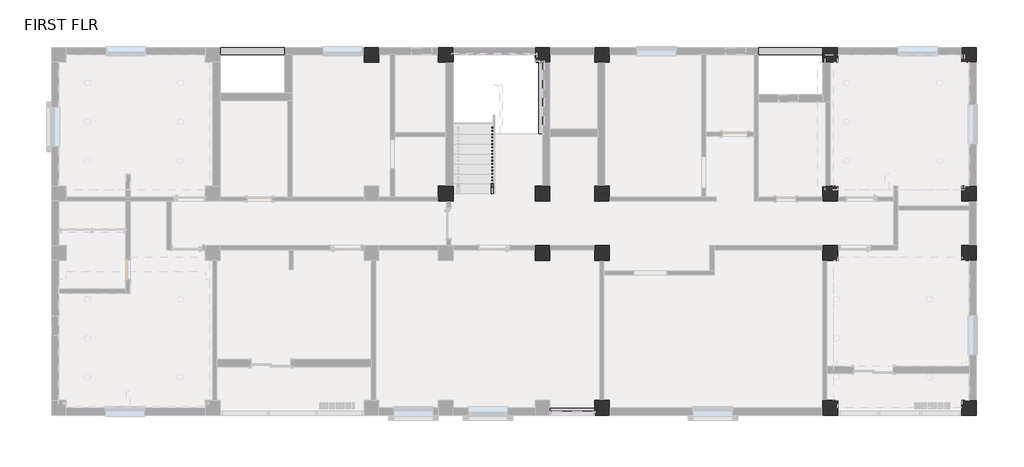
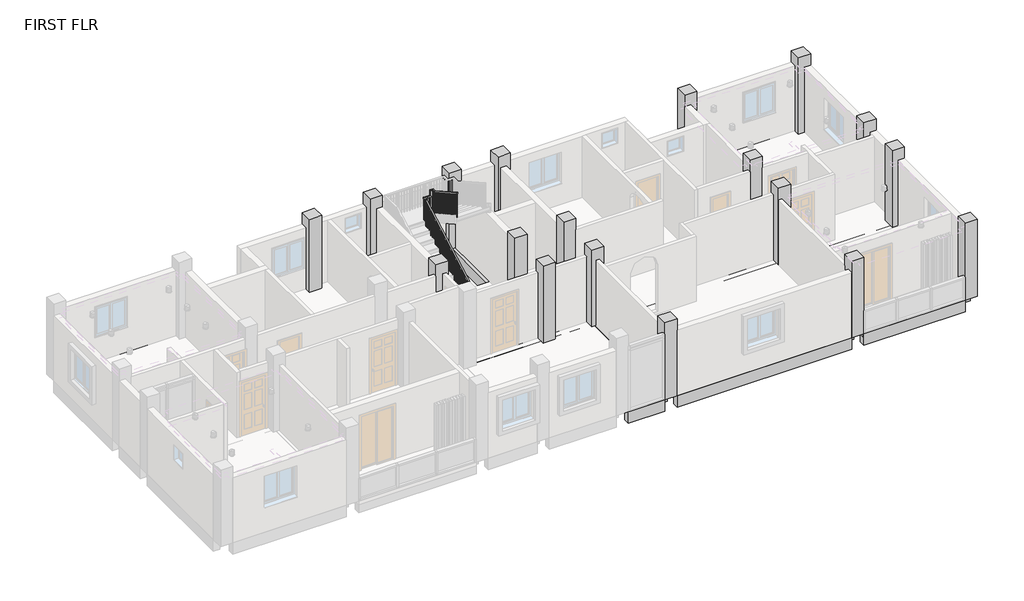
# One storey, part 4 of 5: 32 beams, 18 columns, 1 railing.
"""IFC4 building model written with IfcOpenShell, lengths in millimetres."""

from ifc_helpers import new_model, si_unit, frame, origin, place, context, project, spatial, polyline, outline, extrude, faceted_brep, element, save

model = new_model("IFC4")

# Units and contexts
model_context = context("Model", 3, world=origin())
ifc_project = project(units=[si_unit("LENGTHUNIT", "METRE", prefix="MILLI")], contexts=[model_context])

# Site, building, storey
site = spatial("IfcSite", under=ifc_project)
building = spatial("IfcBuilding", under=site)
storey = spatial("IfcBuildingStorey", under=building, Name="FIRST FLR", Elevation=3352.8)

# Beams
placement = place(None, origin())
element("IfcBeam", 1, ObjectType="Concrete-Rectangular Beam : 9\" X 18\" BEAM", at=placement, inside=storey, context=model_context, shape_type="SweptSolid", body=[
    extrude(outline(polyline([(1310.3916602, -10887.8679047), (1310.3916602, -11116.4679047), (-61.2083398, -11116.4679047), (-61.2083398, -10887.8679047), (1310.3916602, -10887.8679047)])), frame((0.0, 0.0, 2895.6), z_axis=(0.0, 0.0, 1.0), x_axis=(1.0, 0.0, 0.0)), (0.0, 0.0, 1.0), 457.2),
])
element("IfcBeam", 2, ObjectType="Concrete-Rectangular Beam : 9\" X 18\" BEAM", at=placement, inside=storey, context=model_context, shape_type="SweptSolid", body=[
    extrude(outline(polyline([(1424.6916602, -6358.3794704), (1653.2916602, -6358.3794704), (1653.2916602, -10659.2679047), (1424.6916602, -10659.2679047), (1424.6916602, -6358.3794704)])), frame((0.0, 0.0, 2895.6), z_axis=(0.0, 0.0, 1.0), x_axis=(1.0, 0.0, 0.0)), (0.0, 0.0, 1.0), 457.2),
])
element("IfcBeam", 3, ObjectType="Concrete-Rectangular Beam : 9\" X 18\" BEAM", at=placement, inside=storey, context=model_context, shape_type="SweptSolid", body=[
    extrude(outline(polyline([(1424.6916602, -4529.5794704), (1653.2916602, -4529.5794704), (1653.2916602, -5901.1794704), (1424.6916602, -5901.1794704), (1424.6916602, -4529.5794704)])), frame((0.0, 0.0, 2895.6), z_axis=(0.0, 0.0, 1.0), x_axis=(1.0, 0.0, 0.0)), (0.0, 0.0, 1.0), 457.2),
])
element("IfcBeam", 4, ObjectType="Concrete-Rectangular Beam : 9\" X 18\" BEAM", at=placement, inside=storey, context=model_context, shape_type="SweptSolid", body=[
    extrude(outline(polyline([(8317.2128058, -10887.8679047), (8317.2128058, -11116.4679047), (1767.5916602, -11116.4679047), (1767.5916602, -10887.8679047), (8317.2128058, -10887.8679047)])), frame((0.0, 0.0, 2895.6), z_axis=(0.0, 0.0, 1.0), x_axis=(1.0, 0.0, 0.0)), (0.0, 0.0, 1.0), 457.2),
])
element("IfcBeam", 5, ObjectType="Concrete-Rectangular Beam : 9\" X 18\" BEAM", at=placement, inside=storey, context=model_context, shape_type="SweptSolid", body=[
    extrude(outline(polyline([(12584.4128058, -10887.8679047), (12584.4128058, -11116.4679047), (8774.4128058, -11116.4679047), (8774.4128058, -10887.8679047), (12584.4128058, -10887.8679047)])), frame((0.0, 0.0, 2895.6), z_axis=(0.0, 0.0, 1.0), x_axis=(1.0, 0.0, 0.0)), (0.0, 0.0, 1.0), 457.2),
])
element("IfcBeam", 6, ObjectType="Concrete-Rectangular Beam : 9\" X 18\" BEAM", at=placement, inside=storey, context=model_context, shape_type="SweptSolid", body=[
    extrude(outline(polyline([(12813.0128058, -6358.3794704), (13041.6128058, -6358.3794704), (13041.6128058, -10659.2679047), (12813.0128058, -10659.2679047), (12813.0128058, -6358.3794704)])), frame((0.0, 0.0, 2895.6), z_axis=(0.0, 0.0, 1.0), x_axis=(1.0, 0.0, 0.0)), (0.0, 0.0, 1.0), 457.2),
])
element("IfcBeam", 7, ObjectType="Concrete-Rectangular Beam : 9\" X 18\" BEAM", at=placement, inside=storey, context=model_context, shape_type="SweptSolid", body=[
    extrude(outline(polyline([(12813.0128058, -4529.5794704), (13041.6128058, -4529.5794704), (13041.6128058, -5901.1794704), (12813.0128058, -5901.1794704), (12813.0128058, -4529.5794704)])), frame((0.0, 0.0, 2895.6), z_axis=(0.0, 0.0, 1.0), x_axis=(1.0, 0.0, 0.0)), (0.0, 0.0, 1.0), 457.2),
])
element("IfcBeam", 8, ObjectType="Concrete-Rectangular Beam : 9\" X 18\" BEAM", at=placement, inside=storey, context=model_context, shape_type="SweptSolid", body=[
    extrude(outline(polyline([(12813.0128058, -262.3794704), (13041.6128058, -262.3794704), (13041.6128058, -4072.3794704), (12813.0128058, -4072.3794704), (12813.0128058, -262.3794704)])), frame((0.0, 0.0, 2895.6), z_axis=(0.0, 0.0, 1.0), x_axis=(1.0, 0.0, 0.0)), (0.0, 0.0, 1.0), 457.2),
])
element("IfcBeam", 9, ObjectType="Concrete-Rectangular Beam : 9\" X 18\" BEAM", at=placement, inside=storey, context=model_context, shape_type="SweptSolid", body=[
    extrude(outline(polyline([(8774.4128058, -33.7794704), (8774.4128058, 194.8205296), (12584.4128058, 194.8205296), (12584.4128058, -33.7794704), (8774.4128058, -33.7794704)])), frame((0.0, 0.0, 2895.6), z_axis=(0.0, 0.0, 1.0), x_axis=(1.0, 0.0, 0.0)), (0.0, 0.0, 1.0), 457.2),
])
element("IfcBeam", 10, ObjectType="Concrete-Rectangular Beam : 9\" X 18\" BEAM", at=placement, inside=storey, context=model_context, shape_type="SweptSolid", body=[
    extrude(outline(polyline([(1767.5916602, -33.7794704), (1767.5916602, 194.8205296), (8317.2128058, 194.8205296), (8317.2128058, -33.7794704), (1767.5916602, -33.7794704)])), frame((0.0, 0.0, 2895.6), z_axis=(0.0, 0.0, 1.0), x_axis=(1.0, 0.0, 0.0)), (0.0, 0.0, 1.0), 457.2),
])
element("IfcBeam", 11, ObjectType="Concrete-Rectangular Beam : 9\" X 18\" BEAM", at=placement, inside=storey, context=model_context, shape_type="SweptSolid", body=[
    extrude(outline(polyline([(-61.2083398, -33.7794704), (-61.2083398, 194.8205296), (1310.3916602, 194.8205296), (1310.3916602, -33.7794704), (-61.2083398, -33.7794704)])), frame((0.0, 0.0, 2895.6), z_axis=(0.0, 0.0, 1.0), x_axis=(1.0, 0.0, 0.0)), (0.0, 0.0, 1.0), 457.2),
])
element("IfcBeam", 12, ObjectType="Concrete-Rectangular Beam : 9\" X 18\" BEAM", at=placement, inside=storey, context=model_context, shape_type="SweptSolid", body=[
    extrude(outline(polyline([(-3029.5456086, -33.7794704), (-3029.5456086, 194.8205296), (-518.4083398, 194.8205296), (-518.4083398, -33.7794704), (-3029.5456086, -33.7794704)])), frame((0.0, 0.0, 2895.6), z_axis=(0.0, 0.0, 1.0), x_axis=(1.0, 0.0, 0.0)), (0.0, 0.0, 1.0), 457.2),
])
element("IfcBeam", 13, ObjectType="Concrete-Rectangular Beam : 9\" X 18\" BEAM", at=placement, inside=storey, context=model_context, shape_type="SweptSolid", body=[
    extrude(outline(polyline([(-5315.5456086, -33.7794704), (-5315.5456086, 194.8205296), (-3486.7456086, 194.8205296), (-3486.7456086, -33.7794704), (-5315.5456086, -33.7794704)])), frame((0.0, 0.0, 2895.6), z_axis=(0.0, 0.0, 1.0), x_axis=(1.0, 0.0, 0.0)), (0.0, 0.0, 1.0), 457.2),
])
element("IfcBeam", 14, ObjectType="Concrete-Rectangular Beam : 9\" X 18\" BEAM", at=placement, inside=storey, context=model_context, shape_type="SweptSolid", body=[
    extrude(outline(polyline([(-10192.3456086, -33.7794704), (-10192.3456086, 194.8205296), (-5772.7456086, 194.8205296), (-5772.7456086, -33.7794704), (-10192.3456086, -33.7794704)])), frame((0.0, 0.0, 2895.6), z_axis=(0.0, 0.0, 1.0), x_axis=(1.0, 0.0, 0.0)), (0.0, 0.0, 1.0), 457.2),
])
element("IfcBeam", 15, ObjectType="Concrete-Rectangular Beam : 9\" X 18\" BEAM", at=placement, inside=storey, context=model_context, shape_type="SweptSolid", body=[
    extrude(outline(polyline([(-14916.7456086, -33.7794704), (-14916.7456086, 194.8205296), (-10649.5456086, 194.8205296), (-10649.5456086, -33.7794704), (-14916.7456086, -33.7794704)])), frame((0.0, 0.0, 2895.6), z_axis=(0.0, 0.0, 1.0), x_axis=(1.0, 0.0, 0.0)), (0.0, 0.0, 1.0), 457.2),
])
element("IfcBeam", 16, ObjectType="Concrete-Rectangular Beam : 9\" X 18\" BEAM", at=placement, inside=storey, context=model_context, shape_type="SweptSolid", body=[
    extrude(outline(polyline([(-518.4083398, -4186.6794704), (-518.4083398, -4415.2794704), (-3029.5456086, -4415.2794704), (-3029.5456086, -4186.6794704), (-518.4083398, -4186.6794704)])), frame((0.0, 0.0, 2895.6), z_axis=(0.0, 0.0, 1.0), x_axis=(1.0, 0.0, 0.0)), (0.0, 0.0, 1.0), 457.2),
])
element("IfcBeam", 17, ObjectType="Concrete-Rectangular Beam : 9\" X 18\" BEAM", at=placement, inside=storey, context=model_context, shape_type="SweptSolid", body=[
    extrude(outline(polyline([(1310.3916602, -4186.6794704), (1310.3916602, -4415.2794704), (-61.2083398, -4415.2794704), (-61.2083398, -4186.6794704), (1310.3916602, -4186.6794704)])), frame((0.0, 0.0, 2895.6), z_axis=(0.0, 0.0, 1.0), x_axis=(1.0, 0.0, 0.0)), (0.0, 0.0, 1.0), 457.2),
])
element("IfcBeam", 18, ObjectType="Concrete-Rectangular Beam : 9\" X 18\" BEAM", at=placement, inside=storey, context=model_context, shape_type="SweptSolid", body=[
    extrude(outline(polyline([(1424.6916602, -262.3794704), (1653.2916602, -262.3794704), (1653.2916602, -4072.3794704), (1424.6916602, -4072.3794704), (1424.6916602, -262.3794704)])), frame((0.0, 0.0, 2895.6), z_axis=(0.0, 0.0, 1.0), x_axis=(1.0, 0.0, 0.0)), (0.0, 0.0, 1.0), 457.2),
])
element("IfcBeam", 19, ObjectType="Concrete-Rectangular Beam : 9\" X 18\" BEAM", at=placement, inside=storey, context=model_context, shape_type="SweptSolid", body=[
    extrude(outline(polyline([(-175.5083398, -4072.3794704), (-404.1083398, -4072.3794704), (-404.1083398, -262.3794704), (-175.5083398, -262.3794704), (-175.5083398, -4072.3794704)])), frame((0.0, 0.0, 2895.6), z_axis=(0.0, 0.0, 1.0), x_axis=(1.0, 0.0, 0.0)), (0.0, 0.0, 1.0), 457.2),
])
element("IfcBeam", 20, ObjectType="Concrete-Rectangular Beam : 9\" X 18\" BEAM", at=placement, inside=storey, context=model_context, shape_type="SweptSolid", body=[
    extrude(outline(polyline([(-3143.8456086, -4072.3794704), (-3372.4456086, -4072.3794704), (-3372.4456086, -262.3794704), (-3143.8456086, -262.3794704), (-3143.8456086, -4072.3794704)])), frame((0.0, 0.0, 2895.6), z_axis=(0.0, 0.0, 1.0), x_axis=(1.0, 0.0, 0.0)), (0.0, 0.0, 1.0), 457.2),
])
element("IfcBeam", 21, ObjectType="Concrete-Rectangular Beam : 9\" X 18\" BEAM", at=placement, inside=storey, context=model_context, shape_type="SweptSolid", body=[
    extrude(outline(polyline([(-5429.8456086, -4072.3794704), (-5658.4456086, -4072.3794704), (-5658.4456086, -262.3794704), (-5429.8456086, -262.3794704), (-5429.8456086, -4072.3794704)])), frame((0.0, 0.0, 2895.6), z_axis=(0.0, 0.0, 1.0), x_axis=(1.0, 0.0, 0.0)), (0.0, 0.0, 1.0), 457.2),
])
element("IfcBeam", 22, ObjectType="Concrete-Rectangular Beam : 9\" X 18\" BEAM", at=placement, inside=storey, context=model_context, shape_type="SweptSolid", body=[
    extrude(outline(polyline([(-3029.5456086, -6244.0794704), (-3029.5456086, -6015.4794704), (-518.4083398, -6015.4794704), (-518.4083398, -6244.0794704), (-3029.5456086, -6244.0794704)])), frame((0.0, 0.0, 2895.6), z_axis=(0.0, 0.0, 1.0), x_axis=(1.0, 0.0, 0.0)), (0.0, 0.0, 1.0), 457.2),
])
element("IfcBeam", 23, ObjectType="Concrete-Rectangular Beam : 9\" X 18\" BEAM", at=placement, inside=storey, context=model_context, shape_type="SweptSolid", body=[
    extrude(outline(polyline([(1310.3916602, -6015.4794704), (1310.3916602, -6244.0794704), (-61.2083398, -6244.0794704), (-61.2083398, -6015.4794704), (1310.3916602, -6015.4794704)])), frame((0.0, 0.0, 2895.6), z_axis=(0.0, 0.0, 1.0), x_axis=(1.0, 0.0, 0.0)), (0.0, 0.0, 1.0), 457.2),
])
element("IfcBeam", 24, ObjectType="Concrete-Rectangular Beam : 9\" X 18\" BEAM", at=placement, inside=storey, context=model_context, shape_type="SweptSolid", body=[
    extrude(outline(polyline([(-404.1083398, -4529.5794704), (-175.5083398, -4529.5794704), (-175.5083398, -5901.1794704), (-404.1083398, -5901.1794704), (-404.1083398, -4529.5794704)])), frame((0.0, 0.0, 2895.6), z_axis=(0.0, 0.0, 1.0), x_axis=(1.0, 0.0, 0.0)), (0.0, 0.0, 1.0), 457.2),
])
element("IfcBeam", 25, ObjectType="Concrete-Rectangular Beam : 9\" X 18\" BEAM", at=placement, inside=storey, context=model_context, shape_type="SweptSolid", body=[
    extrude(outline(polyline([(-3143.8456086, -5901.1794704), (-3372.4456086, -5901.1794704), (-3372.4456086, -4529.5794704), (-3143.8456086, -4529.5794704), (-3143.8456086, -5901.1794704)])), frame((0.0, 0.0, 2895.6), z_axis=(0.0, 0.0, 1.0), x_axis=(1.0, 0.0, 0.0)), (0.0, 0.0, 1.0), 457.2),
])
element("IfcBeam", 26, ObjectType="Concrete-Rectangular Beam : 9\" X 18\" BEAM", at=placement, inside=storey, context=model_context, shape_type="SweptSolid", body=[
    extrude(outline(polyline([(8317.2128058, -4186.6794704), (8317.2128058, -4415.2794704), (1767.5916602, -4415.2794704), (1767.5916602, -4186.6794704), (8317.2128058, -4186.6794704)])), frame((0.0, 0.0, 2895.6), z_axis=(0.0, 0.0, 1.0), x_axis=(1.0, 0.0, 0.0)), (0.0, 0.0, 1.0), 457.2),
])
element("IfcBeam", 27, ObjectType="Concrete-Rectangular Beam : 9\" X 18\" BEAM", at=placement, inside=storey, context=model_context, shape_type="SweptSolid", body=[
    extrude(outline(polyline([(12584.4128058, -4186.6794704), (12584.4128058, -4415.2794704), (8774.4128058, -4415.2794704), (8774.4128058, -4186.6794704), (12584.4128058, -4186.6794704)])), frame((0.0, 0.0, 2895.6), z_axis=(0.0, 0.0, 1.0), x_axis=(1.0, 0.0, 0.0)), (0.0, 0.0, 1.0), 457.2),
])
element("IfcBeam", 28, ObjectType="Concrete-Rectangular Beam : 9\" X 18\" BEAM", at=placement, inside=storey, context=model_context, shape_type="SweptSolid", body=[
    extrude(outline(polyline([(8774.4128058, -6244.0794704), (8774.4128058, -6015.4794704), (12584.4128058, -6015.4794704), (12584.4128058, -6244.0794704), (8774.4128058, -6244.0794704)])), frame((0.0, 0.0, 2895.6), z_axis=(0.0, 0.0, 1.0), x_axis=(1.0, 0.0, 0.0)), (0.0, 0.0, 1.0), 457.2),
])
element("IfcBeam", 29, ObjectType="Concrete-Rectangular Beam : 9\" X 18\" BEAM", at=placement, inside=storey, context=model_context, shape_type="SweptSolid", body=[
    extrude(outline(polyline([(1767.5916602, -6244.0794704), (1767.5916602, -6015.4794704), (8317.2128058, -6015.4794704), (8317.2128058, -6244.0794704), (1767.5916602, -6244.0794704)])), frame((0.0, 0.0, 2895.6), z_axis=(0.0, 0.0, 1.0), x_axis=(1.0, 0.0, 0.0)), (0.0, 0.0, 1.0), 457.2),
])
element("IfcBeam", 30, ObjectType="Concrete-Rectangular Beam : 9\" X 18\" BEAM", at=placement, inside=storey, context=model_context, shape_type="SweptSolid", body=[
    extrude(outline(polyline([(8431.5128058, -6358.3794704), (8660.1128058, -6358.3794704), (8660.1128058, -10659.2679047), (8431.5128058, -10659.2679047), (8431.5128058, -6358.3794704)])), frame((0.0, 0.0, 2895.6), z_axis=(0.0, 0.0, 1.0), x_axis=(1.0, 0.0, 0.0)), (0.0, 0.0, 1.0), 457.2),
])
element("IfcBeam", 31, ObjectType="Concrete-Rectangular Beam : 9\" X 18\" BEAM", at=placement, inside=storey, context=model_context, shape_type="SweptSolid", body=[
    extrude(outline(polyline([(8431.5128058, -4529.5794704), (8660.1128058, -4529.5794704), (8660.1128058, -5901.1794704), (8431.5128058, -5901.1794704), (8431.5128058, -4529.5794704)])), frame((0.0, 0.0, 2895.6), z_axis=(0.0, 0.0, 1.0), x_axis=(1.0, 0.0, 0.0)), (0.0, 0.0, 1.0), 457.2),
])
element("IfcBeam", 32, ObjectType="Concrete-Rectangular Beam : 9\" X 18\" BEAM", at=placement, inside=storey, context=model_context, shape_type="SweptSolid", body=[
    extrude(outline(polyline([(8431.5128058, -262.3794704), (8660.1128058, -262.3794704), (8660.1128058, -4072.3794704), (8431.5128058, -4072.3794704), (8431.5128058, -262.3794704)])), frame((0.0, 0.0, 2895.6), z_axis=(0.0, 0.0, 1.0), x_axis=(1.0, 0.0, 0.0)), (0.0, 0.0, 1.0), 457.2),
])

# Columns
element("IfcColumn", 33, ObjectType="Concrete-Rectangular-Column : COLUMN 18\" X 18\"", at=placement, inside=storey, context=model_context, shape_type="SweptSolid", body=[
    extrude(outline(polyline([(-5315.5456086, 194.8205296), (-5315.5456086, -262.3794704), (-5772.7456086, -262.3794704), (-5772.7456086, 194.8205296), (-5315.5456086, 194.8205296)])), frame((0.0, 0.0, 3352.8), z_axis=(0.0, 0.0, 1.0), x_axis=(1.0, 0.0, 0.0)), (0.0, 0.0, 1.0), 3048.0),
])
element("IfcColumn", 34, ObjectType="Concrete-Rectangular-Column : COLUMN 18\" X 18\"", at=placement, inside=storey, context=model_context, shape_type="SweptSolid", body=[
    extrude(outline(polyline([(-3029.5456086, 194.8205296), (-3029.5456086, -262.3794704), (-3486.7456086, -262.3794704), (-3486.7456086, 194.8205296), (-3029.5456086, 194.8205296)])), frame((0.0, 0.0, 3352.8), z_axis=(0.0, 0.0, 1.0), x_axis=(1.0, 0.0, 0.0)), (0.0, 0.0, 1.0), 3048.0),
])
element("IfcColumn", 35, ObjectType="Concrete-Rectangular-Column : COLUMN 18\" X 18\"", at=placement, inside=storey, context=model_context, shape_type="SweptSolid", body=[
    extrude(outline(polyline([(-61.2083398, 194.8205296), (-61.2083398, -262.3794704), (-518.4083398, -262.3794704), (-518.4083398, 194.8205296), (-61.2083398, 194.8205296)])), frame((0.0, 0.0, 3352.8), z_axis=(0.0, 0.0, 1.0), x_axis=(1.0, 0.0, 0.0)), (0.0, 0.0, 1.0), 3048.0),
])
element("IfcColumn", 36, ObjectType="Concrete-Rectangular-Column : COLUMN 18\" X 18\"", at=placement, inside=storey, context=model_context, shape_type="SweptSolid", body=[
    extrude(outline(polyline([(1767.5916602, 194.8205296), (1767.5916602, -262.3794704), (1310.3916602, -262.3794704), (1310.3916602, 194.8205296), (1767.5916602, 194.8205296)])), frame((0.0, 0.0, 3352.8), z_axis=(0.0, 0.0, 1.0), x_axis=(1.0, 0.0, 0.0)), (0.0, 0.0, 1.0), 3048.0),
])
element("IfcColumn", 37, ObjectType="Concrete-Rectangular-Column : COLUMN 18\" X 18\"", at=placement, inside=storey, context=model_context, shape_type="SweptSolid", body=[
    extrude(outline(polyline([(8774.4128058, 194.8205296), (8774.4128058, -262.3794704), (8317.2128058, -262.3794704), (8317.2128058, 194.8205296), (8774.4128058, 194.8205296)])), frame((0.0, 0.0, 3352.8), z_axis=(0.0, 0.0, 1.0), x_axis=(1.0, 0.0, 0.0)), (0.0, 0.0, 1.0), 3048.0),
])
element("IfcColumn", 38, ObjectType="Concrete-Rectangular-Column : COLUMN 18\" X 18\"", at=placement, inside=storey, context=model_context, shape_type="SweptSolid", body=[
    extrude(outline(polyline([(13041.6128058, 194.8205296), (13041.6128058, -262.3794704), (12584.4128058, -262.3794704), (12584.4128058, 194.8205296), (13041.6128058, 194.8205296)])), frame((0.0, 0.0, 3352.8), z_axis=(0.0, 0.0, 1.0), x_axis=(1.0, 0.0, 0.0)), (0.0, 0.0, 1.0), 3048.0),
])
element("IfcColumn", 39, ObjectType="Concrete-Rectangular-Column : COLUMN 18\" X 18\"", at=placement, inside=storey, context=model_context, shape_type="SweptSolid", body=[
    extrude(outline(polyline([(13041.6128058, -4072.3794704), (13041.6128058, -4529.5794704), (12584.4128058, -4529.5794704), (12584.4128058, -4072.3794704), (13041.6128058, -4072.3794704)])), frame((0.0, 0.0, 3352.8), z_axis=(0.0, 0.0, 1.0), x_axis=(1.0, 0.0, 0.0)), (0.0, 0.0, 1.0), 3048.0),
])
element("IfcColumn", 40, ObjectType="Concrete-Rectangular-Column : COLUMN 18\" X 18\"", at=placement, inside=storey, context=model_context, shape_type="SweptSolid", body=[
    extrude(outline(polyline([(13041.6128058, -5901.1794704), (13041.6128058, -6358.3794704), (12584.4128058, -6358.3794704), (12584.4128058, -5901.1794704), (13041.6128058, -5901.1794704)])), frame((0.0, 0.0, 3352.8), z_axis=(0.0, 0.0, 1.0), x_axis=(1.0, 0.0, 0.0)), (0.0, 0.0, 1.0), 3048.0),
])
element("IfcColumn", 41, ObjectType="Concrete-Rectangular-Column : COLUMN 18\" X 18\"", at=placement, inside=storey, context=model_context, shape_type="SweptSolid", body=[
    extrude(outline(polyline([(13041.6128058, -10659.2679047), (13041.6128058, -11116.4679047), (12584.4128058, -11116.4679047), (12584.4128058, -10659.2679047), (13041.6128058, -10659.2679047)])), frame((0.0, 0.0, 3352.8), z_axis=(0.0, 0.0, 1.0), x_axis=(1.0, 0.0, 0.0)), (0.0, 0.0, 1.0), 3048.0),
])
element("IfcColumn", 42, ObjectType="Concrete-Rectangular-Column : COLUMN 18\" X 18\"", at=placement, inside=storey, context=model_context, shape_type="SweptSolid", body=[
    extrude(outline(polyline([(8774.4128058, -10659.2679047), (8774.4128058, -11116.4679047), (8317.2128058, -11116.4679047), (8317.2128058, -10659.2679047), (8774.4128058, -10659.2679047)])), frame((0.0, 0.0, 3352.8), z_axis=(0.0, 0.0, 1.0), x_axis=(1.0, 0.0, 0.0)), (0.0, 0.0, 1.0), 3048.0),
])
element("IfcColumn", 43, ObjectType="Concrete-Rectangular-Column : COLUMN 18\" X 18\"", at=placement, inside=storey, context=model_context, shape_type="SweptSolid", body=[
    extrude(outline(polyline([(1767.5916602, -10659.2679047), (1767.5916602, -11116.4679047), (1310.3916602, -11116.4679047), (1310.3916602, -10659.2679047), (1767.5916602, -10659.2679047)])), frame((0.0, 0.0, 3352.8), z_axis=(0.0, 0.0, 1.0), x_axis=(1.0, 0.0, 0.0)), (0.0, 0.0, 1.0), 3048.0),
])
element("IfcColumn", 44, ObjectType="Concrete-Rectangular-Column : COLUMN 18\" X 18\"", at=placement, inside=storey, context=model_context, shape_type="SweptSolid", body=[
    extrude(outline(polyline([(-3029.5456086, -4072.3794704), (-3029.5456086, -4529.5794704), (-3486.7456086, -4529.5794704), (-3486.7456086, -4072.3794704), (-3029.5456086, -4072.3794704)])), frame((0.0, 0.0, 3352.8), z_axis=(0.0, 0.0, 1.0), x_axis=(1.0, 0.0, 0.0)), (0.0, 0.0, 1.0), 3048.0),
])
element("IfcColumn", 45, ObjectType="Concrete-Rectangular-Column : COLUMN 18\" X 18\"", at=placement, inside=storey, context=model_context, shape_type="SweptSolid", body=[
    extrude(outline(polyline([(-61.2083398, -4072.3794704), (-61.2083398, -4529.5794704), (-518.4083398, -4529.5794704), (-518.4083398, -4072.3794704), (-61.2083398, -4072.3794704)])), frame((0.0, 0.0, 3352.8), z_axis=(0.0, 0.0, 1.0), x_axis=(1.0, 0.0, 0.0)), (0.0, 0.0, 1.0), 3048.0),
])
element("IfcColumn", 46, ObjectType="Concrete-Rectangular-Column : COLUMN 18\" X 18\"", at=placement, inside=storey, context=model_context, shape_type="SweptSolid", body=[
    extrude(outline(polyline([(1767.5916602, -4072.3794704), (1767.5916602, -4529.5794704), (1310.3916602, -4529.5794704), (1310.3916602, -4072.3794704), (1767.5916602, -4072.3794704)])), frame((0.0, 0.0, 3352.8), z_axis=(0.0, 0.0, 1.0), x_axis=(1.0, 0.0, 0.0)), (0.0, 0.0, 1.0), 3048.0),
])
element("IfcColumn", 47, ObjectType="Concrete-Rectangular-Column : COLUMN 18\" X 18\"", at=placement, inside=storey, context=model_context, shape_type="SweptSolid", body=[
    extrude(outline(polyline([(8774.4128058, -4072.3794704), (8774.4128058, -4529.5794704), (8317.2128058, -4529.5794704), (8317.2128058, -4072.3794704), (8774.4128058, -4072.3794704)])), frame((0.0, 0.0, 3352.8), z_axis=(0.0, 0.0, 1.0), x_axis=(1.0, 0.0, 0.0)), (0.0, 0.0, 1.0), 3048.0),
])
element("IfcColumn", 48, ObjectType="Concrete-Rectangular-Column : COLUMN 18\" X 18\"", at=placement, inside=storey, context=model_context, shape_type="SweptSolid", body=[
    extrude(outline(polyline([(8774.4128058, -5901.1794704), (8774.4128058, -6358.3794704), (8317.2128058, -6358.3794704), (8317.2128058, -5901.1794704), (8774.4128058, -5901.1794704)])), frame((0.0, 0.0, 3352.8), z_axis=(0.0, 0.0, 1.0), x_axis=(1.0, 0.0, 0.0)), (0.0, 0.0, 1.0), 3048.0),
])
element("IfcColumn", 49, ObjectType="Concrete-Rectangular-Column : COLUMN 18\" X 18\"", at=placement, inside=storey, context=model_context, shape_type="SweptSolid", body=[
    extrude(outline(polyline([(1767.5916602, -5901.1794704), (1767.5916602, -6358.3794704), (1310.3916602, -6358.3794704), (1310.3916602, -5901.1794704), (1767.5916602, -5901.1794704)])), frame((0.0, 0.0, 3352.8), z_axis=(0.0, 0.0, 1.0), x_axis=(1.0, 0.0, 0.0)), (0.0, 0.0, 1.0), 3048.0),
])
element("IfcColumn", 50, ObjectType="Concrete-Rectangular-Column : COLUMN 18\" X 18\"", at=placement, inside=storey, context=model_context, shape_type="SweptSolid", body=[
    extrude(outline(polyline([(-61.2083398, -5901.1794704), (-61.2083398, -6358.3794704), (-518.4083398, -6358.3794704), (-518.4083398, -5901.1794704), (-61.2083398, -5901.1794704)])), frame((0.0, 0.0, 3352.8), z_axis=(0.0, 0.0, 1.0), x_axis=(1.0, 0.0, 0.0)), (0.0, 0.0, 1.0), 3048.0),
])

# Railing
element("IfcRailing", 51, ObjectType="Handrail - Rectangular", at=placement, inside=storey, context=model_context, shape_type="SolidModel", body=[
    faceted_brep([(-1861.1456086, -4300.9794704, 4436.5333333), (-1861.1456086, -4300.9794704, 4378.420221), (-1810.3456086, -4300.9794704, 4378.420221), (-1810.3456086, -4300.9794704, 4436.5333333), (-1861.1456086, -1024.3794704, 6256.8666667), (-1861.1456086, -973.5794704, 6226.9757765), (-1810.3456086, -973.5794704, 6226.9757765), (-1810.3456086, -1024.3794704, 6256.8666667), (-1861.1456086, -1024.3794704, 6299.2), (-1861.1456086, -973.5794704, 6248.4), (-1810.3456086, -973.5794704, 6248.4), (-1810.3456086, -1024.3794704, 6299.2), (-1861.1456086, -897.3794704, 6299.2), (-1861.1456086, -897.3794704, 6248.4), (-1810.3456086, -948.1794704, 6248.4), (-1810.3456086, -948.1794704, 6299.2), (-1734.1456086, -897.3794704, 6299.2), (-1734.1456086, -897.3794704, 6248.4), (-1734.1456086, -948.1794704, 6248.4), (-1734.1456086, -948.1794704, 6299.2), (-1610.6083398, -897.3794704, 6299.2), (-1559.8083398, -897.3794704, 6248.4), (-1559.8083398, -948.1794704, 6248.4), (-1610.6083398, -948.1794704, 6299.2), (-1610.6083398, -897.3794704, 6510.8666667), (-1559.8083398, -897.3794704, 6460.0666667), (-1559.8083398, -948.1794704, 6460.0666667), (-1610.6083398, -948.1794704, 6510.8666667), (-1483.6083398, -897.3794704, 6510.8666667), (-1483.6083398, -897.3794704, 6460.0666667), (-1534.4083398, -948.1794704, 6460.0666667), (-1534.4083398, -948.1794704, 6510.8666667), (-1483.6083398, -1024.3794704, 6510.8666667), (-1483.6083398, -1037.5430727, 6460.0666667), (-1534.4083398, -1037.5430727, 6460.0666667), (-1534.4083398, -1024.3794704, 6510.8666667), (-1483.6083398, -2472.1794704, 7315.2), (-1534.4083398, -2472.1794704, 7315.2), (-1534.4083398, -2472.1794704, 7257.0868876), (-1483.6083398, -2472.1794704, 7257.0868876)], [[[0, 1, 2, 3]], [[1, 0, 4, 5]], [[2, 1, 5, 6]], [[3, 2, 6, 7]], [[0, 3, 7, 4]], [[5, 4, 8, 9]], [[6, 5, 9, 10]], [[7, 6, 10, 11]], [[4, 7, 11, 8]], [[9, 8, 12, 13]], [[10, 9, 13, 14]], [[11, 10, 14, 15]], [[8, 11, 15, 12]], [[13, 12, 16, 17]], [[14, 13, 17, 18]], [[15, 14, 18, 19]], [[12, 15, 19, 16]], [[17, 16, 20, 21]], [[18, 17, 21, 22]], [[19, 18, 22, 23]], [[16, 19, 23, 20]], [[21, 20, 24, 25]], [[22, 21, 25, 26]], [[23, 22, 26, 27]], [[20, 23, 27, 24]], [[25, 24, 28, 29]], [[26, 25, 29, 30]], [[27, 26, 30, 31]], [[24, 27, 31, 28]], [[29, 28, 32, 33]], [[30, 29, 33, 34]], [[31, 30, 34, 35]], [[28, 31, 35, 32]], [[36, 37, 38, 39]], [[33, 32, 36, 39]], [[34, 33, 39, 38]], [[35, 34, 38, 37]], [[32, 35, 37, 36]]]),
    extrude(outline(polyline([(-2456.3044704, 7248.2674432), (-2437.2544704, 7237.6841099), (-2437.2544704, 6231.4666667), (-2456.3044704, 6231.4666667), (-2456.3044704, 7248.2674432)])), frame((-1518.5333398, 0.0, 0.0), z_axis=(1.0, 0.0, 0.0), x_axis=(0.0, 1.0, 0.0)), (0.0, 0.0, 1.0), 19.05),
    extrude(outline(polyline([(-2354.7044704, 7191.8229988), (-2335.6544704, 7181.2396654), (-2335.6544704, 6231.4666667), (-2354.7044704, 6231.4666667), (-2354.7044704, 7191.8229988)])), frame((-1518.5333398, 0.0, 0.0), z_axis=(1.0, 0.0, 0.0), x_axis=(0.0, 1.0, 0.0)), (0.0, 0.0, 1.0), 19.05),
    extrude(outline(polyline([(-2253.1044704, 7135.3785543), (-2234.0544704, 7124.795221), (-2234.0544704, 6231.4666667), (-2253.1044704, 6231.4666667), (-2253.1044704, 7135.3785543)])), frame((-1518.5333398, 0.0, 0.0), z_axis=(1.0, 0.0, 0.0), x_axis=(0.0, 1.0, 0.0)), (0.0, 0.0, 1.0), 19.05),
    extrude(outline(polyline([(-2151.5044704, 7078.9341099), (-2132.4544704, 7068.3507765), (-2132.4544704, 6062.1333333), (-2151.5044704, 6062.1333333), (-2151.5044704, 7078.9341099)])), frame((-1518.5333398, 0.0, 0.0), z_axis=(1.0, 0.0, 0.0), x_axis=(0.0, 1.0, 0.0)), (0.0, 0.0, 1.0), 19.05),
    extrude(outline(polyline([(-2049.9044704, 7022.4896654), (-2030.8544704, 7011.9063321), (-2030.8544704, 6062.1333333), (-2049.9044704, 6062.1333333), (-2049.9044704, 7022.4896654)])), frame((-1518.5333398, 0.0, 0.0), z_axis=(1.0, 0.0, 0.0), x_axis=(0.0, 1.0, 0.0)), (0.0, 0.0, 1.0), 19.05),
    extrude(outline(polyline([(-1948.3044704, 6966.045221), (-1929.2544704, 6955.4618876), (-1929.2544704, 6062.1333333), (-1948.3044704, 6062.1333333), (-1948.3044704, 6966.045221)])), frame((-1518.5333398, 0.0, 0.0), z_axis=(1.0, 0.0, 0.0), x_axis=(0.0, 1.0, 0.0)), (0.0, 0.0, 1.0), 19.05),
    extrude(outline(polyline([(-1846.7044704, 6909.6007765), (-1827.6544704, 6899.0174432), (-1827.6544704, 5892.8), (-1846.7044704, 5892.8), (-1846.7044704, 6909.6007765)])), frame((-1518.5333398, 0.0, 0.0), z_axis=(1.0, 0.0, 0.0), x_axis=(0.0, 1.0, 0.0)), (0.0, 0.0, 1.0), 19.05),
    extrude(outline(polyline([(-1745.1044704, 6853.1563321), (-1726.0544704, 6842.5729988), (-1726.0544704, 5892.8), (-1745.1044704, 5892.8), (-1745.1044704, 6853.1563321)])), frame((-1518.5333398, 0.0, 0.0), z_axis=(1.0, 0.0, 0.0), x_axis=(0.0, 1.0, 0.0)), (0.0, 0.0, 1.0), 19.05),
    extrude(outline(polyline([(-1643.5044704, 6796.7118876), (-1624.4544704, 6786.1285543), (-1624.4544704, 5892.8), (-1643.5044704, 5892.8), (-1643.5044704, 6796.7118876)])), frame((-1518.5333398, 0.0, 0.0), z_axis=(1.0, 0.0, 0.0), x_axis=(0.0, 1.0, 0.0)), (0.0, 0.0, 1.0), 19.05),
    extrude(outline(polyline([(-1541.9044704, 6740.2674432), (-1522.8544704, 6729.6841099), (-1522.8544704, 5723.4666667), (-1541.9044704, 5723.4666667), (-1541.9044704, 6740.2674432)])), frame((-1518.5333398, 0.0, 0.0), z_axis=(1.0, 0.0, 0.0), x_axis=(0.0, 1.0, 0.0)), (0.0, 0.0, 1.0), 19.05),
    extrude(outline(polyline([(-1440.3044704, 6683.8229988), (-1421.2544704, 6673.2396654), (-1421.2544704, 5723.4666667), (-1440.3044704, 5723.4666667), (-1440.3044704, 6683.8229988)])), frame((-1518.5333398, 0.0, 0.0), z_axis=(1.0, 0.0, 0.0), x_axis=(0.0, 1.0, 0.0)), (0.0, 0.0, 1.0), 19.05),
    extrude(outline(polyline([(-1338.7044704, 6627.3785543), (-1319.6544704, 6616.795221), (-1319.6544704, 5723.4666667), (-1338.7044704, 5723.4666667), (-1338.7044704, 6627.3785543)])), frame((-1518.5333398, 0.0, 0.0), z_axis=(1.0, 0.0, 0.0), x_axis=(0.0, 1.0, 0.0)), (0.0, 0.0, 1.0), 19.05),
    extrude(outline(polyline([(-1237.1044704, 6570.9341099), (-1218.0544704, 6560.3507765), (-1218.0544704, 5554.1333333), (-1237.1044704, 5554.1333333), (-1237.1044704, 6570.9341099)])), frame((-1518.5333398, 0.0, 0.0), z_axis=(1.0, 0.0, 0.0), x_axis=(0.0, 1.0, 0.0)), (0.0, 0.0, 1.0), 19.05),
    extrude(outline(polyline([(-1135.5044704, 6514.4896654), (-1116.4544704, 6503.9063321), (-1116.4544704, 5554.1333333), (-1135.5044704, 5554.1333333), (-1135.5044704, 6514.4896654)])), frame((-1518.5333398, 0.0, 0.0), z_axis=(1.0, 0.0, 0.0), x_axis=(0.0, 1.0, 0.0)), (0.0, 0.0, 1.0), 19.05),
    extrude(outline(polyline([(-1033.9044704, 6458.045221), (-1014.8544704, 6447.4618876), (-1014.8544704, 5554.1333333), (-1033.9044704, 5554.1333333), (-1033.9044704, 6458.045221)])), frame((-1518.5333398, 0.0, 0.0), z_axis=(1.0, 0.0, 0.0), x_axis=(0.0, 1.0, 0.0)), (0.0, 0.0, 1.0), 19.05),
    extrude(outline(polyline([(-1540.4706086, -932.3044704), (-1540.4706086, -913.2544704), (-1521.4206086, -913.2544704), (-1521.4206086, -932.3044704), (-1540.4706086, -932.3044704)])), frame((0.0, 0.0, 5384.8), z_axis=(0.0, 0.0, 1.0), x_axis=(1.0, 0.0, 0.0)), (0.0, 0.0, 1.0), 1075.2666667),
    extrude(outline(polyline([(-1642.0706086, -932.3044704), (-1642.0706086, -913.2544704), (-1623.0206086, -913.2544704), (-1623.0206086, -932.3044704), (-1642.0706086, -932.3044704)])), frame((0.0, 0.0, 5384.8), z_axis=(0.0, 0.0, 1.0), x_axis=(1.0, 0.0, 0.0)), (0.0, 0.0, 1.0), 863.6),
    extrude(outline(polyline([(-1743.6706086, -932.3044704), (-1743.6706086, -913.2544704), (-1724.6206086, -913.2544704), (-1724.6206086, -932.3044704), (-1743.6706086, -932.3044704)])), frame((0.0, 0.0, 5384.8), z_axis=(0.0, 0.0, 1.0), x_axis=(1.0, 0.0, 0.0)), (0.0, 0.0, 1.0), 863.6),
    extrude(outline(polyline([(-1826.2206086, -957.7044704), (-1845.2706086, -957.7044704), (-1845.2706086, -938.6544704), (-1826.2206086, -938.6544704), (-1826.2206086, -957.7044704)])), frame((0.0, 0.0, 5384.8), z_axis=(0.0, 0.0, 1.0), x_axis=(1.0, 0.0, 0.0)), (0.0, 0.0, 1.0), 863.6),
    extrude(outline(polyline([(-1059.3044704, 6179.3507765), (-1040.2544704, 6189.9341099), (-1040.2544704, 5215.4666667), (-1059.3044704, 5215.4666667), (-1059.3044704, 6179.3507765)])), frame((-1845.2706086, 0.0, 0.0), z_axis=(1.0, 0.0, 0.0), x_axis=(0.0, 1.0, 0.0)), (0.0, 0.0, 1.0), 19.05),
    extrude(outline(polyline([(-1160.9044704, 6122.9063321), (-1141.8544704, 6133.4896654), (-1141.8544704, 5215.4666667), (-1160.9044704, 5215.4666667), (-1160.9044704, 6122.9063321)])), frame((-1845.2706086, 0.0, 0.0), z_axis=(1.0, 0.0, 0.0), x_axis=(0.0, 1.0, 0.0)), (0.0, 0.0, 1.0), 19.05),
    extrude(outline(polyline([(-1262.5044704, 6066.4618876), (-1243.4544704, 6077.045221), (-1243.4544704, 5215.4666667), (-1262.5044704, 5215.4666667), (-1262.5044704, 6066.4618876)])), frame((-1845.2706086, 0.0, 0.0), z_axis=(1.0, 0.0, 0.0), x_axis=(0.0, 1.0, 0.0)), (0.0, 0.0, 1.0), 19.05),
    extrude(outline(polyline([(-1364.1044704, 6010.0174432), (-1345.0544704, 6020.6007765), (-1345.0544704, 5046.1333333), (-1364.1044704, 5046.1333333), (-1364.1044704, 6010.0174432)])), frame((-1845.2706086, 0.0, 0.0), z_axis=(1.0, 0.0, 0.0), x_axis=(0.0, 1.0, 0.0)), (0.0, 0.0, 1.0), 19.05),
    extrude(outline(polyline([(-1465.7044704, 5953.5729988), (-1446.6544704, 5964.1563321), (-1446.6544704, 5046.1333333), (-1465.7044704, 5046.1333333), (-1465.7044704, 5953.5729988)])), frame((-1845.2706086, 0.0, 0.0), z_axis=(1.0, 0.0, 0.0), x_axis=(0.0, 1.0, 0.0)), (0.0, 0.0, 1.0), 19.05),
    extrude(outline(polyline([(-1567.3044704, 5897.1285543), (-1548.2544704, 5907.7118876), (-1548.2544704, 5046.1333333), (-1567.3044704, 5046.1333333), (-1567.3044704, 5897.1285543)])), frame((-1845.2706086, 0.0, 0.0), z_axis=(1.0, 0.0, 0.0), x_axis=(0.0, 1.0, 0.0)), (0.0, 0.0, 1.0), 19.05),
    extrude(outline(polyline([(-1668.9044704, 5840.6841099), (-1649.8544704, 5851.2674432), (-1649.8544704, 4876.8), (-1668.9044704, 4876.8), (-1668.9044704, 5840.6841099)])), frame((-1845.2706086, 0.0, 0.0), z_axis=(1.0, 0.0, 0.0), x_axis=(0.0, 1.0, 0.0)), (0.0, 0.0, 1.0), 19.05),
    extrude(outline(polyline([(-1770.5044704, 5784.2396654), (-1751.4544704, 5794.8229988), (-1751.4544704, 4876.8), (-1770.5044704, 4876.8), (-1770.5044704, 5784.2396654)])), frame((-1845.2706086, 0.0, 0.0), z_axis=(1.0, 0.0, 0.0), x_axis=(0.0, 1.0, 0.0)), (0.0, 0.0, 1.0), 19.05),
    extrude(outline(polyline([(-1872.1044704, 5727.795221), (-1853.0544704, 5738.3785543), (-1853.0544704, 4876.8), (-1872.1044704, 4876.8), (-1872.1044704, 5727.795221)])), frame((-1845.2706086, 0.0, 0.0), z_axis=(1.0, 0.0, 0.0), x_axis=(0.0, 1.0, 0.0)), (0.0, 0.0, 1.0), 19.05),
    extrude(outline(polyline([(-1973.7044704, 5671.3507765), (-1954.6544704, 5681.9341099), (-1954.6544704, 4707.4666667), (-1973.7044704, 4707.4666667), (-1973.7044704, 5671.3507765)])), frame((-1845.2706086, 0.0, 0.0), z_axis=(1.0, 0.0, 0.0), x_axis=(0.0, 1.0, 0.0)), (0.0, 0.0, 1.0), 19.05),
    extrude(outline(polyline([(-2075.3044704, 5614.9063321), (-2056.2544704, 5625.4896654), (-2056.2544704, 4707.4666667), (-2075.3044704, 4707.4666667), (-2075.3044704, 5614.9063321)])), frame((-1845.2706086, 0.0, 0.0), z_axis=(1.0, 0.0, 0.0), x_axis=(0.0, 1.0, 0.0)), (0.0, 0.0, 1.0), 19.05),
    extrude(outline(polyline([(-2176.9044704, 5558.4618876), (-2157.8544704, 5569.045221), (-2157.8544704, 4707.4666667), (-2176.9044704, 4707.4666667), (-2176.9044704, 5558.4618876)])), frame((-1845.2706086, 0.0, 0.0), z_axis=(1.0, 0.0, 0.0), x_axis=(0.0, 1.0, 0.0)), (0.0, 0.0, 1.0), 19.05),
    extrude(outline(polyline([(-2278.5044704, 5502.0174432), (-2259.4544704, 5512.6007765), (-2259.4544704, 4538.1333333), (-2278.5044704, 4538.1333333), (-2278.5044704, 5502.0174432)])), frame((-1845.2706086, 0.0, 0.0), z_axis=(1.0, 0.0, 0.0), x_axis=(0.0, 1.0, 0.0)), (0.0, 0.0, 1.0), 19.05),
    extrude(outline(polyline([(-2380.1044704, 5445.5729988), (-2361.0544704, 5456.1563321), (-2361.0544704, 4538.1333333), (-2380.1044704, 4538.1333333), (-2380.1044704, 5445.5729988)])), frame((-1845.2706086, 0.0, 0.0), z_axis=(1.0, 0.0, 0.0), x_axis=(0.0, 1.0, 0.0)), (0.0, 0.0, 1.0), 19.05),
    extrude(outline(polyline([(-2481.7044704, 5389.1285543), (-2462.6544704, 5399.7118876), (-2462.6544704, 4538.1333333), (-2481.7044704, 4538.1333333), (-2481.7044704, 5389.1285543)])), frame((-1845.2706086, 0.0, 0.0), z_axis=(1.0, 0.0, 0.0), x_axis=(0.0, 1.0, 0.0)), (0.0, 0.0, 1.0), 19.05),
    extrude(outline(polyline([(-2583.3044704, 5332.6841099), (-2564.2544704, 5343.2674432), (-2564.2544704, 4368.8), (-2583.3044704, 4368.8), (-2583.3044704, 5332.6841099)])), frame((-1845.2706086, 0.0, 0.0), z_axis=(1.0, 0.0, 0.0), x_axis=(0.0, 1.0, 0.0)), (0.0, 0.0, 1.0), 19.05),
    extrude(outline(polyline([(-2684.9044704, 5276.2396654), (-2665.8544704, 5286.8229988), (-2665.8544704, 4368.8), (-2684.9044704, 4368.8), (-2684.9044704, 5276.2396654)])), frame((-1845.2706086, 0.0, 0.0), z_axis=(1.0, 0.0, 0.0), x_axis=(0.0, 1.0, 0.0)), (0.0, 0.0, 1.0), 19.05),
    extrude(outline(polyline([(-2786.5044704, 5219.795221), (-2767.4544704, 5230.3785543), (-2767.4544704, 4368.8), (-2786.5044704, 4368.8), (-2786.5044704, 5219.795221)])), frame((-1845.2706086, 0.0, 0.0), z_axis=(1.0, 0.0, 0.0), x_axis=(0.0, 1.0, 0.0)), (0.0, 0.0, 1.0), 19.05),
    extrude(outline(polyline([(-2888.1044704, 5163.3507765), (-2869.0544704, 5173.9341099), (-2869.0544704, 4199.4666667), (-2888.1044704, 4199.4666667), (-2888.1044704, 5163.3507765)])), frame((-1845.2706086, 0.0, 0.0), z_axis=(1.0, 0.0, 0.0), x_axis=(0.0, 1.0, 0.0)), (0.0, 0.0, 1.0), 19.05),
    extrude(outline(polyline([(-2989.7044704, 5106.9063321), (-2970.6544704, 5117.4896654), (-2970.6544704, 4199.4666667), (-2989.7044704, 4199.4666667), (-2989.7044704, 5106.9063321)])), frame((-1845.2706086, 0.0, 0.0), z_axis=(1.0, 0.0, 0.0), x_axis=(0.0, 1.0, 0.0)), (0.0, 0.0, 1.0), 19.05),
    extrude(outline(polyline([(-3091.3044704, 5050.4618876), (-3072.2544704, 5061.045221), (-3072.2544704, 4199.4666667), (-3091.3044704, 4199.4666667), (-3091.3044704, 5050.4618876)])), frame((-1845.2706086, 0.0, 0.0), z_axis=(1.0, 0.0, 0.0), x_axis=(0.0, 1.0, 0.0)), (0.0, 0.0, 1.0), 19.05),
    extrude(outline(polyline([(-3192.9044704, 4994.0174432), (-3173.8544704, 5004.6007765), (-3173.8544704, 4030.1333333), (-3192.9044704, 4030.1333333), (-3192.9044704, 4994.0174432)])), frame((-1845.2706086, 0.0, 0.0), z_axis=(1.0, 0.0, 0.0), x_axis=(0.0, 1.0, 0.0)), (0.0, 0.0, 1.0), 19.05),
    extrude(outline(polyline([(-3294.5044704, 4937.5729988), (-3275.4544704, 4948.1563321), (-3275.4544704, 4030.1333333), (-3294.5044704, 4030.1333333), (-3294.5044704, 4937.5729988)])), frame((-1845.2706086, 0.0, 0.0), z_axis=(1.0, 0.0, 0.0), x_axis=(0.0, 1.0, 0.0)), (0.0, 0.0, 1.0), 19.05),
    extrude(outline(polyline([(-3396.1044704, 4881.1285543), (-3377.0544704, 4891.7118876), (-3377.0544704, 4030.1333333), (-3396.1044704, 4030.1333333), (-3396.1044704, 4881.1285543)])), frame((-1845.2706086, 0.0, 0.0), z_axis=(1.0, 0.0, 0.0), x_axis=(0.0, 1.0, 0.0)), (0.0, 0.0, 1.0), 19.05),
    extrude(outline(polyline([(-3497.7044704, 4824.6841099), (-3478.6544704, 4835.2674432), (-3478.6544704, 3860.8), (-3497.7044704, 3860.8), (-3497.7044704, 4824.6841099)])), frame((-1845.2706086, 0.0, 0.0), z_axis=(1.0, 0.0, 0.0), x_axis=(0.0, 1.0, 0.0)), (0.0, 0.0, 1.0), 19.05),
    extrude(outline(polyline([(-3599.3044704, 4768.2396654), (-3580.2544704, 4778.8229988), (-3580.2544704, 3860.8), (-3599.3044704, 3860.8), (-3599.3044704, 4768.2396654)])), frame((-1845.2706086, 0.0, 0.0), z_axis=(1.0, 0.0, 0.0), x_axis=(0.0, 1.0, 0.0)), (0.0, 0.0, 1.0), 19.05),
    extrude(outline(polyline([(-3700.9044704, 4711.795221), (-3681.8544704, 4722.3785543), (-3681.8544704, 3860.8), (-3700.9044704, 3860.8), (-3700.9044704, 4711.795221)])), frame((-1845.2706086, 0.0, 0.0), z_axis=(1.0, 0.0, 0.0), x_axis=(0.0, 1.0, 0.0)), (0.0, 0.0, 1.0), 19.05),
    extrude(outline(polyline([(-3802.5044704, 4655.3507765), (-3783.4544704, 4665.9341099), (-3783.4544704, 3691.4666667), (-3802.5044704, 3691.4666667), (-3802.5044704, 4655.3507765)])), frame((-1845.2706086, 0.0, 0.0), z_axis=(1.0, 0.0, 0.0), x_axis=(0.0, 1.0, 0.0)), (0.0, 0.0, 1.0), 19.05),
    extrude(outline(polyline([(-3904.1044704, 4598.9063321), (-3885.0544704, 4609.4896654), (-3885.0544704, 3691.4666667), (-3904.1044704, 3691.4666667), (-3904.1044704, 4598.9063321)])), frame((-1845.2706086, 0.0, 0.0), z_axis=(1.0, 0.0, 0.0), x_axis=(0.0, 1.0, 0.0)), (0.0, 0.0, 1.0), 19.05),
    extrude(outline(polyline([(-4005.7044704, 4542.4618876), (-3986.6544704, 4553.045221), (-3986.6544704, 3691.4666667), (-4005.7044704, 3691.4666667), (-4005.7044704, 4542.4618876)])), frame((-1845.2706086, 0.0, 0.0), z_axis=(1.0, 0.0, 0.0), x_axis=(0.0, 1.0, 0.0)), (0.0, 0.0, 1.0), 19.05),
    extrude(outline(polyline([(-4107.3044704, 4486.0174432), (-4088.2544704, 4496.6007765), (-4088.2544704, 3522.1333333), (-4107.3044704, 3522.1333333), (-4107.3044704, 4486.0174432)])), frame((-1845.2706086, 0.0, 0.0), z_axis=(1.0, 0.0, 0.0), x_axis=(0.0, 1.0, 0.0)), (0.0, 0.0, 1.0), 19.05),
    extrude(outline(polyline([(-4208.9044704, 4429.5729988), (-4189.8544704, 4440.1563321), (-4189.8544704, 3522.1333333), (-4208.9044704, 3522.1333333), (-4208.9044704, 4429.5729988)])), frame((-1845.2706086, 0.0, 0.0), z_axis=(1.0, 0.0, 0.0), x_axis=(0.0, 1.0, 0.0)), (0.0, 0.0, 1.0), 19.05),
    extrude(outline(polyline([(-1518.5333398, -932.3044704), (-1518.5333398, -913.2544704), (-1499.4833398, -913.2544704), (-1499.4833398, -932.3044704), (-1518.5333398, -932.3044704)])), frame((0.0, 0.0, 5384.8), z_axis=(0.0, 0.0, 1.0), x_axis=(1.0, 0.0, 0.0)), (0.0, 0.0, 1.0), 1075.2666667),
    extrude(outline(polyline([(-1826.2206086, -932.3044704), (-1845.2706086, -932.3044704), (-1845.2706086, -913.2544704), (-1826.2206086, -913.2544704), (-1826.2206086, -932.3044704)])), frame((0.0, 0.0, 5384.8), z_axis=(0.0, 0.0, 1.0), x_axis=(1.0, 0.0, 0.0)), (0.0, 0.0, 1.0), 863.6),
    extrude(outline(polyline([(-2472.1794704, 7257.0868876), (-2453.1294704, 7246.5035543), (-2453.1294704, 6231.4666667), (-2472.1794704, 6231.4666667), (-2472.1794704, 7257.0868876)])), frame((-1518.5333398, 0.0, 0.0), z_axis=(1.0, 0.0, 0.0), x_axis=(0.0, 1.0, 0.0)), (0.0, 0.0, 1.0), 19.05),
    extrude(outline(polyline([(-4300.9794704, 4378.420221), (-4281.9294704, 4389.0035543), (-4281.9294704, 3522.1333333), (-4300.9794704, 3522.1333333), (-4300.9794704, 4378.420221)])), frame((-1845.2706086, 0.0, 0.0), z_axis=(1.0, 0.0, 0.0), x_axis=(0.0, 1.0, 0.0)), (0.0, 0.0, 1.0), 19.05),
])

save(model, "model.ifc")

# Revit data of these elements
# Type "Concrete-Rectangular Beam : 9\" X 18\" BEAM"
#   Assembly Code = "B10"
#   Length [instance default] = 5' - 0"
#   b = 0' - 9"
#   h = 1' - 6"
#   Structural Material [instance default] = Concrete, Cast-in-Place gray
# Type "Concrete-Rectangular-Column : COLUMN 18\" X 18\""
#   Assembly Code = "B10"
#   b = 1' - 6"
#   h = 1' - 6"
#   Structural Material [instance default] = Concrete, Cast-in-Place gray
# Type "Handrail - Rectangular"
#   Assembly Code = "C2010400"
#   built-in parameter 1008612 = 0.0416667 (stored number, unit not read)
#   built-in parameter 1008611 = 0.0416667 (stored number, unit not read)
#   built-in parameter 1008609 = 0.333333 (stored number, unit not read)
#   built-in parameter 1008604 = 0.166667 (stored number, unit not read)
#   built-in parameter 1008603 = 0.166667 (stored number, unit not read)
#   Railing Height = 3' - 0"
#   built-in parameter 1008630 = 2
#   built-in parameter 1008610 = 2
#   built-in parameter 1008618 = Baluster - Square : 3/4"
# Elements 1, 4, 5, 6, 7, 8, 9, 10, 11, 12, 13, 15 (IfcBeam, "Concrete-Rectangular Beam : 9\" X 18\" BEAM")
#   Structural Material = Concrete, Cast-in-Place gray
#   Phase Created = New Construction
#   Materials on its faces: "Concrete, Cast-in-Place gray", "SAND BEIGE PAINT"
# Elements 2, 3, 16, 17, 18, 19, 20, 21, 22, 23, 24, 25, 26, 27, 28, 29, 30, 31, 32 (IfcBeam, "Concrete-Rectangular Beam : 9\" X 18\" BEAM")
#   Structural Material = Concrete, Cast-in-Place gray
#   Phase Created = New Construction
#   Materials on its faces: "Concrete, Cast-in-Place gray"
# Element 14 (IfcBeam, "Concrete-Rectangular Beam : 9\" X 18\" BEAM")
#   Structural Material = Concrete, Cast-in-Place gray
#   Phase Created = New Construction
#   Materials on its faces: "SAND BEIGE PAINT", "Concrete, Cast-in-Place gray"
# Elements 33, 34, 35, 36, 37, 38, 39, 40, 41, 42, 43 (IfcColumn, "Concrete-Rectangular-Column : COLUMN 18\" X 18\"")
#   Structural Material = Concrete, Cast-in-Place gray
#   Phase Created = New Construction
#   Materials on its faces: "Concrete, Cast-in-Place gray", "SAND BEIGE PAINT"
# Elements 44, 45, 46, 47, 48, 49, 50 (IfcColumn, "Concrete-Rectangular-Column : COLUMN 18\" X 18\"")
#   Structural Material = Concrete, Cast-in-Place gray
#   Phase Created = New Construction
#   Materials on its faces: "Concrete, Cast-in-Place gray"
# Element 51 (IfcRailing, "Handrail - Rectangular")
#   Phase Created = New Construction
# Materials
#   "Concrete, Cast-in-Place gray": class "Concrete", colour RGB 192 192 192, transparency 0, Description = "Cast-in-place concrete", Cost = 0
#   "SAND BEIGE PAINT": class "Generic", colour RGB 120 120 120, transparency 0, Cost = 0
